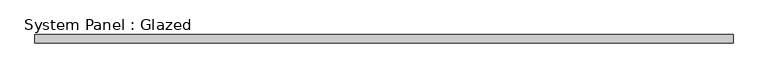
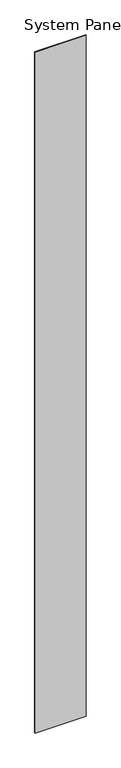
"""IFC4 building model written with IfcOpenShell, lengths in millimetres: plate geometry, System Panel : Glazed."""

from ifc_helpers import new_model, si_unit, origin, origin_with_axes, place, context, project, spatial, polyline, outline, extrude, source, transform, mapped, element, save


def system_panel_glazed_b656db30(model_context):
    return source(origin(), model_context, "Body", "SweptSolid", [
        extrude(outline(polyline([(1035.05, 19.05), (-1035.05, 19.05), (-1035.05, 44.45), (1035.05, 44.45), (1035.05, 19.05)])), origin_with_axes(), (0.0, 0.0, 1.0), 29133.8),
    ])


if __name__ == "__main__":
    model = new_model("IFC4")
    model_context = context("Model", 3, world=origin())
    ifc_project = project(units=[si_unit("LENGTHUNIT", "METRE", prefix="MILLI")], contexts=[model_context])
    site = spatial("IfcSite", under=ifc_project)
    building = spatial("IfcBuilding", under=site)
    placement = place(None, origin())
    system_panel_glazed_shape = system_panel_glazed_b656db30(model_context)
    element("IfcPlate", 1, ObjectType="System Panel : Glazed", at=placement, inside=building, context=model_context, shape_type="MappedRepresentation", body=[
        mapped(system_panel_glazed_shape, transform((0.0, 0.0, 0.0), x_axis=(1.0, 0.0, 0.0), y_axis=(0.0, 1.0, 0.0), z_axis=(0.0, 0.0, 1.0))),
    ])
    save(model, "model.ifc")

# Revit data of these elements
# Type "System Panel : Glazed"
#   Construction Type Id = "GSP4R"
#   Analytic Construction = "1/8 in Pilkington single glazing"
#   Visual Light Transmittance = 0.9
#   Solar Heat Gain Coefficient = 0.86
#   Heat Transfer Coefficient (U) = 1.18115 BTU/(h·ft²·°F)
# Element 1 (IfcPlate, "System Panel : Glazed")
#   Materials on its faces: "Glass"
# Materials
#   "Glass": class "Glass", colour RGB 0 128 192, transparency 0.75, Description = "Soda Lime Glass", Cost = 0
